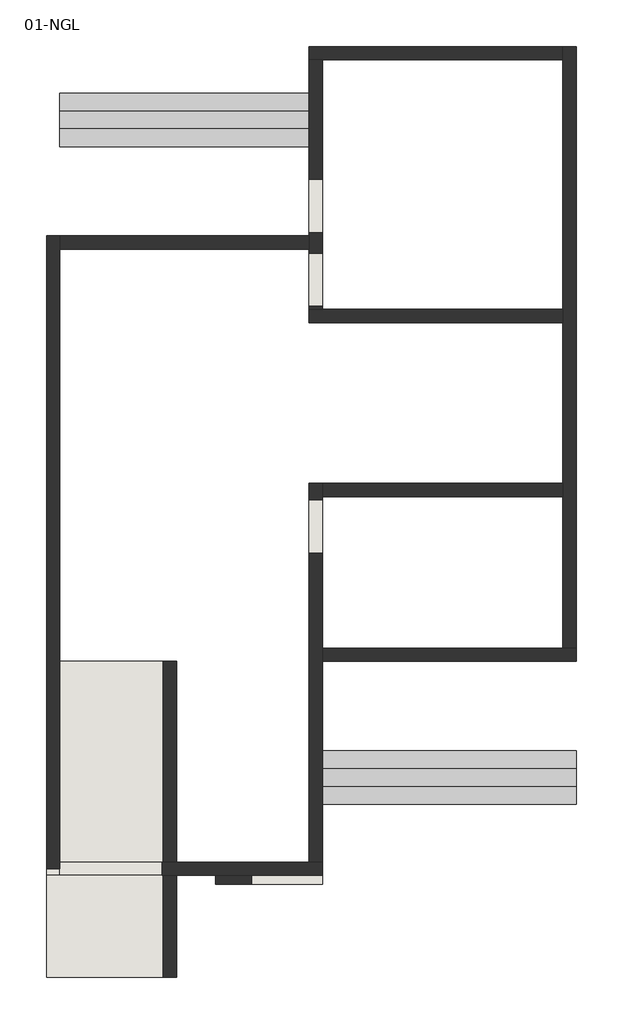
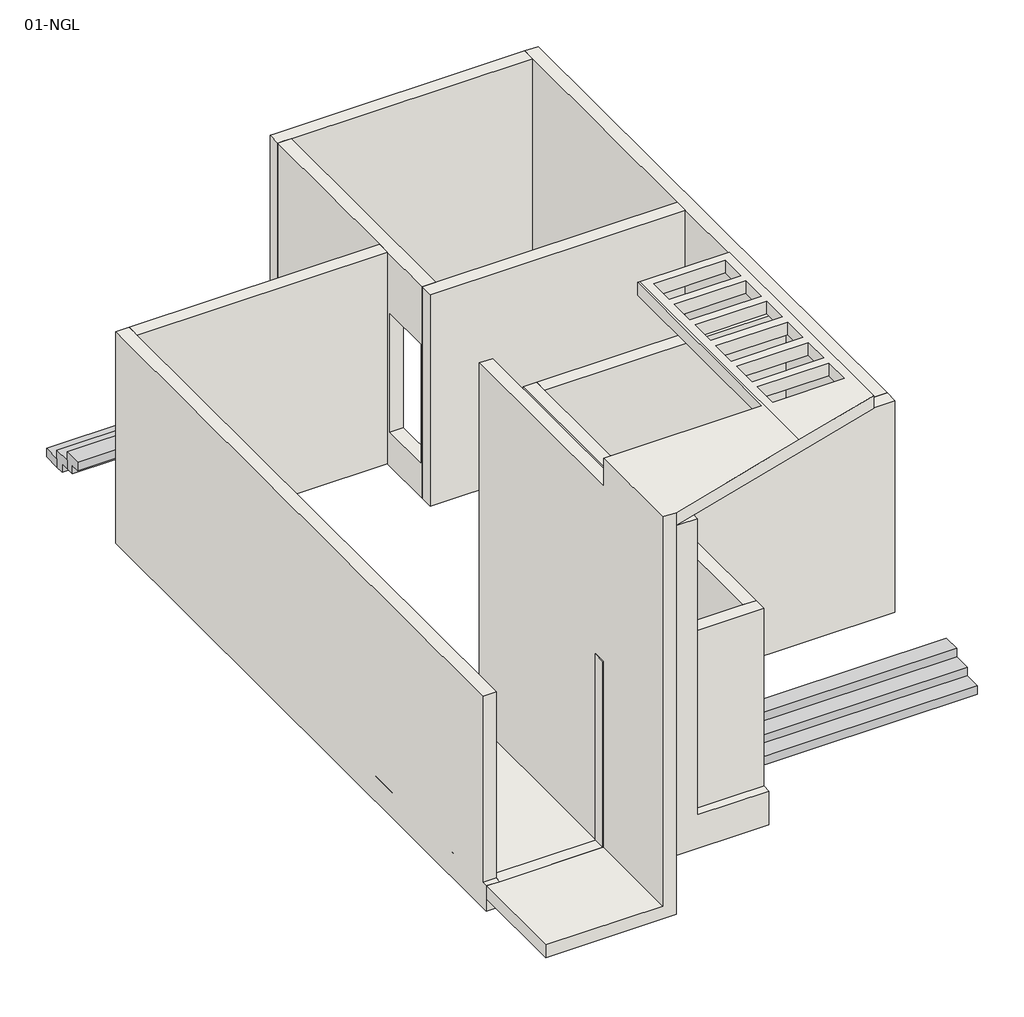
# One storey: 12 walls, 2 stair flights.
"""IFC4 building model written with IfcOpenShell, lengths in millimetres."""

from ifc_helpers import new_model, si_unit, origin, origin_with_axes, place, context, project, spatial, polyline, outline, extrude, faceted_brep, transform, mapped, element, save
from components import walls_1_walls_1_280b9ad2

model = new_model("IFC4")

# Units and contexts
model_context = context("Model", 3, world=origin())
ifc_project = project(units=[si_unit("LENGTHUNIT", "METRE", prefix="MILLI")], contexts=[model_context])

# Site, building, storey
site = spatial("IfcSite", under=ifc_project)
building = spatial("IfcBuilding", under=site)
storey = spatial("IfcBuildingStorey", under=building, Name="01-NGL", Elevation=0.0)

# Stair flights
placement = place(None, origin())
element("IfcStairFlight", 1, ObjectType="01-steps", at=placement, inside=storey, context=model_context, shape_type="Brep", body=[
    faceted_brep([(-9917.6792561, -4576.7197682, 150.0), (-9917.6792561, -4876.7197682, 150.0), (-5642.6792561, -4876.7197682, 150.0), (-5642.6792561, -4576.7197682, 150.0), (-9917.6792561, -4576.7197682, 0.0), (-9917.6792561, -4876.7197682, 0.0), (-5642.6792561, -4876.7197682, 0.0), (-5642.6792561, -4576.7197682, 0.0), (-9917.6792561, -4276.7197682, 300.0), (-9917.6792561, -4576.7197682, 300.0), (-5642.6792561, -4576.7197682, 300.0), (-5642.6792561, -4276.7197682, 300.0), (-9917.6792561, -4276.7197682, 150.0), (-9917.6792561, -4426.7197682, 150.0), (-9917.6792561, -4426.7197682, 0.0), (-5642.6792561, -4426.7197682, 0.0), (-5642.6792561, -4426.7197682, 150.0), (-5642.6792561, -4276.7197682, 150.0), (-9917.6792561, -3976.7197682, 450.0), (-9917.6792561, -4276.7197682, 450.0), (-5642.6792561, -4276.7197682, 450.0), (-5642.6792561, -3976.7197682, 450.0), (-9917.6792561, -3976.7197682, 300.0), (-9917.6792561, -4126.7197682, 300.0), (-9917.6792561, -4126.7197682, 150.0), (-5642.6792561, -4126.7197682, 150.0), (-5642.6792561, -4126.7197682, 300.0), (-5642.6792561, -3976.7197682, 300.0)], [[[0, 1, 2, 3]], [[1, 0, 4, 5]], [[2, 1, 5, 6]], [[3, 2, 6, 7]], [[8, 9, 10, 11]], [[4, 0, 9, 8, 12, 13, 14]], [[0, 3, 10, 9]], [[3, 7, 15, 16, 17, 11, 10]], [[18, 19, 20, 21]], [[19, 18, 22, 23, 24, 12, 8]], [[8, 11, 20, 19]], [[21, 20, 11, 17, 25, 26, 27]], [[18, 21, 27, 22]], [[5, 4, 14, 15, 7, 6]], [[13, 16, 15, 14]], [[24, 25, 17, 16, 13, 12]], [[25, 24, 23, 26]], [[26, 23, 22, 27]]]),
])
element("IfcStairFlight", 2, ObjectType="01-steps", at=placement, inside=storey, context=model_context, shape_type="Brep", body=[
    faceted_brep([(-10142.6792561, 6788.2802318, 150.0), (-10142.6792561, 7088.2802318, 150.0), (-14342.6792561, 7088.2802318, 150.0), (-14342.6792561, 6788.2802318, 150.0), (-14342.6792561, 7088.2802318, 0.0), (-14342.6792561, 6788.2802318, 0.0), (-10142.6792561, 7088.2802318, 0.0), (-10142.6792561, 6788.2802318, 0.0), (-10142.6792561, 6488.2802318, 300.0), (-10142.6792561, 6788.2802318, 300.0), (-14342.6792561, 6788.2802318, 300.0), (-14342.6792561, 6488.2802318, 300.0), (-14342.6792561, 6638.2802318, 0.0), (-14342.6792561, 6638.2802318, 150.0), (-14342.6792561, 6488.2802318, 150.0), (-10142.6792561, 6488.2802318, 150.0), (-10142.6792561, 6638.2802318, 150.0), (-10142.6792561, 6638.2802318, 0.0), (-10142.6792561, 6188.2802318, 450.0), (-10142.6792561, 6488.2802318, 450.0), (-14342.6792561, 6488.2802318, 450.0), (-14342.6792561, 6188.2802318, 450.0), (-14342.6792561, 6338.2802318, 150.0), (-14342.6792561, 6338.2802318, 300.0), (-14342.6792561, 6188.2802318, 300.0), (-10142.6792561, 6188.2802318, 300.0), (-10142.6792561, 6338.2802318, 300.0), (-10142.6792561, 6338.2802318, 150.0)], [[[0, 1, 2, 3]], [[3, 2, 4, 5]], [[2, 1, 6, 4]], [[1, 0, 7, 6]], [[8, 9, 10, 11]], [[3, 5, 12, 13, 14, 11, 10]], [[0, 3, 10, 9]], [[7, 0, 9, 8, 15, 16, 17]], [[18, 19, 20, 21]], [[21, 20, 11, 14, 22, 23, 24]], [[8, 11, 20, 19]], [[19, 18, 25, 26, 27, 15, 8]], [[18, 21, 24, 25]], [[6, 7, 17, 12, 5, 4]], [[16, 13, 12, 17]], [[27, 22, 14, 13, 16, 15]], [[22, 27, 26, 23]], [[23, 26, 25, 24]]]),
])

# Walls
element("IfcWall", 3, ObjectType="01-225 WALL", at=placement, inside=storey, context=model_context, shape_type="Brep", body=[
    faceted_brep([(-14567.6792561, 4688.2802318, 3750.0), (-14567.6792561, 4688.2802318, 3300.0), (-14567.6792561, 4688.2802318, 0.0), (-14567.6792561, -6069.2197682, 0.0), (-14567.6792561, -6069.2197682, 450.0), (-14567.6792561, -5964.2197682, 450.0), (-14567.6792561, -5964.2197682, 3750.0), (-14567.6792561, -5851.7197682, 3750.0), (-14567.6792561, 4575.7802318, 3750.0), (-14342.6792561, 4688.2802318, 0.0), (-14342.6792561, 4688.2802318, 3300.0), (-14342.6792561, 4688.2802318, 3750.0), (-14342.6792561, 4575.7802318, 3750.0), (-14342.6792561, 4463.2802318, 3750.0), (-14342.6792561, -5851.7197682, 3750.0), (-14342.6792561, -5964.2197682, 3750.0), (-14342.6792561, -5964.2197682, 450.0), (-14342.6792561, -6069.2197682, 450.0), (-14342.6792561, -6069.2197682, 0.0), (-14342.6792561, -5859.2197682, 0.0), (-14342.6792561, 4463.2802318, 0.0)], [[[0, 1, 2, 3, 4, 5, 6, 7, 8]], [[9, 10, 11, 12, 13, 14, 15, 16, 17, 18, 19, 20]], [[3, 2, 9, 20, 19, 18]], [[0, 8, 7, 6, 15, 14, 13, 12, 11]], [[0, 11, 10, 9, 2, 1]], [[6, 5, 16, 15]], [[16, 5, 4, 17]], [[4, 3, 18, 17]]]),
])
element("IfcWall", 4, ObjectType="01-225 WALL", at=placement, inside=storey, context=model_context, shape_type="Brep", body=[
    faceted_brep([(-12617.6792561, -6076.7197682, 0.0), (-9917.6792561, -6076.7197682, 0.0), (-9917.6792561, -6076.7197682, 3750.0), (-12617.6792561, -6076.7197682, 3750.0), (-12617.6792561, -5851.7197682, 0.0), (-12617.6792561, -5851.7197682, 450.0), (-12617.6792561, -5851.7197682, 3750.0), (-10142.6792561, -5851.7197682, 3750.0), (-9917.6792561, -5851.7197682, 3750.0), (-9917.6792561, -5851.7197682, 0.0), (-10142.6792561, -5851.7197682, 0.0)], [[[0, 1, 2, 3]], [[4, 5, 6, 7, 8, 9, 10]], [[1, 0, 4, 10, 9]], [[3, 2, 8, 7, 6]], [[2, 1, 9, 8]], [[0, 3, 6, 5, 4]]]),
])
element("IfcWall", 5, ObjectType="01-225 WALL", at=placement, inside=storey, context=model_context, shape_type="Brep", body=[
    faceted_brep([(-9917.6792561, -5851.7197682, 0.0), (-9917.6792561, -2476.7197682, 0.0), (-9917.6792561, -2251.7197682, 0.0), (-9917.6792561, 298.2802318, 0.0), (-9917.6792561, 523.2802318, 0.0), (-9917.6792561, 523.2802318, 3750.0), (-9917.6792561, 298.2802318, 3750.0), (-9917.6792561, -2251.7197682, 3750.0), (-9917.6792561, -2476.7197682, 3750.0), (-9917.6792561, -5851.7197682, 3750.0), (-9917.6792561, 248.2802318, 600.0), (-9917.6792561, -651.7197682, 600.0), (-9917.6792561, -651.7197682, 2700.0), (-9917.6792561, 248.2802318, 2700.0), (-10142.6792561, -5851.7197682, 0.0), (-10142.6792561, -5851.7197682, 3750.0), (-10142.6792561, 523.2802318, 3750.0), (-10142.6792561, 523.2802318, 0.0), (-10142.6792561, 248.2802318, 600.0), (-10142.6792561, 248.2802318, 2700.0), (-10142.6792561, -651.7197682, 2700.0), (-10142.6792561, -651.7197682, 600.0)], [[[0, 1, 2, 3, 4, 5, 6, 7, 8, 9], [10, 11, 12, 13]], [[14, 15, 16, 17], [18, 19, 20, 21]], [[4, 3, 2, 1, 0, 14, 17]], [[9, 8, 7, 6, 5, 16, 15]], [[0, 9, 15, 14]], [[5, 4, 17, 16]], [[19, 18, 10, 13]], [[20, 19, 13, 12]], [[21, 20, 12, 11]], [[18, 21, 11, 10]]]),
])
element("IfcWall", 6, ObjectType="01-225 WALL", at=placement, inside=storey, context=model_context, shape_type="Brep", body=[
    faceted_brep([(-9917.6792561, -2476.7197682, 0.0), (-5642.6792561, -2476.7197682, 0.0), (-5642.6792561, -2476.7197682, 3750.0), (-9917.6792561, -2476.7197682, 3750.0), (-9917.6792561, -2251.7197682, 0.0), (-9917.6792561, -2251.7197682, 3750.0), (-5867.6792561, -2251.7197682, 3750.0), (-5642.6792561, -2251.7197682, 3750.0), (-5642.6792561, -2251.7197682, 0.0), (-5867.6792561, -2251.7197682, 0.0)], [[[0, 1, 2, 3]], [[4, 5, 6, 7, 8, 9]], [[1, 0, 4, 9, 8]], [[3, 2, 7, 6, 5]], [[0, 3, 5, 4]], [[2, 1, 8, 7]]]),
])
element("IfcWall", 7, ObjectType="01-225 WALL", at=placement, inside=storey, context=model_context, shape_type="Brep", body=[
    faceted_brep([(-5642.6792561, -2251.7197682, 0.0), (-5642.6792561, 7873.2802318, 0.0), (-5642.6792561, 7873.2802318, 3750.0), (-5642.6792561, -2251.7197682, 3750.0), (-5867.6792561, -2251.7197682, 0.0), (-5867.6792561, -2251.7197682, 3750.0), (-5867.6792561, 298.2802318, 3750.0), (-5867.6792561, 523.2802318, 3750.0), (-5867.6792561, 3223.2802318, 3750.0), (-5867.6792561, 3448.2802318, 3750.0), (-5867.6792561, 7648.2802318, 3750.0), (-5867.6792561, 7873.2802318, 3750.0), (-5867.6792561, 7873.2802318, 0.0), (-5867.6792561, 7648.2802318, 0.0), (-5867.6792561, 3448.2802318, 0.0), (-5867.6792561, 3223.2802318, 0.0), (-5867.6792561, 523.2802318, 0.0), (-5867.6792561, 298.2802318, 0.0)], [[[0, 1, 2, 3]], [[4, 5, 6, 7, 8, 9, 10, 11, 12, 13, 14, 15, 16, 17]], [[1, 0, 4, 17, 16, 15, 14, 13, 12]], [[3, 2, 11, 10, 9, 8, 7, 6, 5]], [[0, 3, 5, 4]], [[2, 1, 12, 11]]]),
])
element("IfcWall", 8, ObjectType="01-225 WALL", at=placement, inside=storey, context=model_context, shape_type="Brep", body=[
    faceted_brep([(-5867.6792561, 7873.2802318, 0.0), (-10142.6792561, 7873.2802318, 0.0), (-10142.6792561, 7873.2802318, 3300.0), (-10142.6792561, 7873.2802318, 3750.0), (-10030.1792561, 7873.2802318, 3750.0), (-5867.6792561, 7873.2802318, 3750.0), (-5867.6792561, 7648.2802318, 0.0), (-5867.6792561, 7648.2802318, 3750.0), (-9917.6792561, 7648.2802318, 3750.0), (-10030.1792561, 7648.2802318, 3750.0), (-10142.6792561, 7648.2802318, 3750.0), (-10142.6792561, 7648.2802318, 3300.0), (-10142.6792561, 7648.2802318, 0.0), (-9917.6792561, 7648.2802318, 0.0)], [[[0, 1, 2, 3, 4, 5]], [[6, 7, 8, 9, 10, 11, 12, 13]], [[1, 0, 6, 13, 12]], [[5, 4, 3, 10, 9, 8, 7]], [[0, 5, 7, 6]], [[1, 12, 11, 10, 3, 2]]]),
])
element("IfcWall", 9, ObjectType="01-225 WALL", at=placement, inside=storey, context=model_context, shape_type="SweptSolid", body=[
    extrude(outline(polyline([(-14342.6792561, 4688.2802318), (-10142.6792561, 4688.2802318), (-10142.6792561, 4463.2802318), (-14342.6792561, 4463.2802318), (-14342.6792561, 4688.2802318)])), origin_with_axes(), (0.0, 0.0, 1.0), 3750.0),
])
element("IfcWall", 10, ObjectType="01-225 WALL", at=placement, inside=storey, context=model_context, shape_type="SweptSolid", body=[
    extrude(outline(polyline([(-5867.6792561, 298.2802318), (-9917.6792561, 298.2802318), (-9917.6792561, 523.2802318), (-5867.6792561, 523.2802318), (-5867.6792561, 298.2802318)])), origin_with_axes(), (0.0, 0.0, 1.0), 3750.0),
])
element("IfcWall", 11, ObjectType="01-225 WALL", at=placement, inside=storey, context=model_context, shape_type="Brep", body=[
    faceted_brep([(-10142.6792561, 3223.2802318, 0.0), (-5867.6792561, 3223.2802318, 0.0), (-5867.6792561, 3223.2802318, 3750.0), (-10142.6792561, 3223.2802318, 3750.0), (-10142.6792561, 3448.2802318, 0.0), (-10142.6792561, 3448.2802318, 3750.0), (-9917.6792561, 3448.2802318, 3750.0), (-5867.6792561, 3448.2802318, 3750.0), (-5867.6792561, 3448.2802318, 0.0), (-9917.6792561, 3448.2802318, 0.0)], [[[0, 1, 2, 3]], [[4, 5, 6, 7, 8, 9]], [[1, 0, 4, 9, 8]], [[3, 2, 7, 6, 5]], [[2, 1, 8, 7]], [[0, 3, 5, 4]]]),
])
element("IfcWall", 12, ObjectType="01-225 WALL", at=placement, inside=storey, context=model_context, shape_type="Brep", body=[
    faceted_brep([(-9917.6792561, 3448.2802318, 0.0), (-9917.6792561, 7648.2802318, 0.0), (-9917.6792561, 7648.2802318, 3750.0), (-9917.6792561, 3448.2802318, 3750.0), (-9917.6792561, 3498.2802318, 2700.0), (-9917.6792561, 4398.2802318, 2700.0), (-9917.6792561, 4398.2802318, 600.0), (-9917.6792561, 3498.2802318, 600.0), (-9917.6792561, 4738.2802318, 600.0), (-9917.6792561, 4738.2802318, 2700.0), (-9917.6792561, 5638.2802318, 2700.0), (-9917.6792561, 5638.2802318, 600.0), (-10142.6792561, 7648.2802318, 0.0), (-10142.6792561, 4688.2802318, 0.0), (-10142.6792561, 4463.2802318, 0.0), (-10142.6792561, 3448.2802318, 0.0), (-10142.6792561, 3448.2802318, 3750.0), (-10142.6792561, 4463.2802318, 3750.0), (-10142.6792561, 4688.2802318, 3750.0), (-10142.6792561, 7648.2802318, 3750.0), (-10142.6792561, 4398.2802318, 2700.0), (-10142.6792561, 3498.2802318, 2700.0), (-10142.6792561, 3498.2802318, 600.0), (-10142.6792561, 4398.2802318, 600.0), (-10142.6792561, 4738.2802318, 2700.0), (-10142.6792561, 4738.2802318, 600.0), (-10142.6792561, 5638.2802318, 600.0), (-10142.6792561, 5638.2802318, 2700.0)], [[[0, 1, 2, 3], [4, 5, 6, 7], [8, 9, 10, 11]], [[12, 13, 14, 15, 16, 17, 18, 19], [20, 21, 22, 23], [24, 25, 26, 27]], [[1, 0, 15, 14, 13, 12]], [[3, 2, 19, 18, 17, 16]], [[0, 3, 16, 15]], [[4, 21, 20, 5]], [[5, 20, 23, 6]], [[6, 23, 22, 7]], [[21, 4, 7, 22]], [[9, 8, 25, 24]], [[10, 9, 24, 27]], [[11, 10, 27, 26]], [[8, 11, 26, 25]], [[1, 12, 19, 2]]]),
])
element("IfcWall", 13, ObjectType="01-225 WALL MAIN", at=placement, inside=storey, context=model_context, shape_type="Brep", body=[
    faceted_brep([(-12617.6792561, -5859.2197682, 0.0), (-14342.6792561, -5859.2197682, 0.0), (-14342.6792561, -5859.2197682, 450.0), (-12617.6792561, -5859.2197682, 450.0), (-12617.6792561, -6069.2197682, 0.0), (-12617.6792561, -6069.2197682, 450.0), (-14342.6792561, -6069.2197682, 450.0), (-14342.6792561, -6069.2197682, 0.0), (-14342.6792561, -5964.2197682, 450.0)], [[[0, 1, 2, 3]], [[4, 5, 6, 7]], [[1, 0, 4, 7]], [[3, 2, 8, 6, 5]], [[0, 3, 5, 4]], [[2, 1, 7, 6, 8]]]),
])
walls_1_walls_1_shape = walls_1_walls_1_280b9ad2(model_context)
element("IfcWall", 14, ObjectType="Walls 1 : Walls 1", at=placement, inside=storey, context=model_context, shape_type="MappedRepresentation", body=[
    mapped(walls_1_walls_1_shape, transform((0.0, 0.0, 0.0), x_axis=(1.0, 0.0, 0.0), y_axis=(0.0, 1.0, 0.0), z_axis=(0.0, 0.0, 1.0))),
])

save(model, "model.ifc")

# Revit data of these elements
# Type "01-225 WALL"
#   Description = "Generic Wall (Material By Category), 200mm thick"
#   Assembly Code = "B2010"
#   Type Mark = "G06"
#   Layers, outside or top first: 225 mm no material (function 1)
# Type "01-225 WALL MAIN"
#   Description = "Generic Wall (Material By Category), 200mm thick"
#   Assembly Code = "B2010"
#   Type Mark = "G06"
#   Layers, outside or top first: 5 mm "01-WHITE WALL PAINT" (function 4); 200 mm "01-DEFAULT WALL" (function 1); 5 mm "01-WHITE WALL PAINT" (function 5)
# Elements 1, 2 (IfcStairFlight, "01-steps")
#   Phase Created = New Construction
# Element 3 (IfcWall, "01-225 WALL")
#   Top Offset = 0 mm
#   Base Offset = 0 mm
#   wall height = 3750 mm
#   Phase Created = New Construction
#   Base Constraint = 01-NGL
#   Top Constraint = 04-FIRST FLOOR
#   Materials on its faces: "Default Wall", "01-WHITE WALL PAINT"
# Elements 4, 5, 6, 7, 8, 9, 10, 11, 12 (IfcWall, "01-225 WALL")
#   Top Offset = 0 mm
#   Base Offset = 0 mm
#   wall height = 3750 mm
#   Phase Created = New Construction
#   Base Constraint = 01-NGL
#   Top Constraint = 04-FIRST FLOOR
#   Materials on its faces: "Default Wall"
# Element 13 (IfcWall, "01-225 WALL MAIN")
#   Top Offset = -150 mm
#   Base Offset = 0 mm
#   wall height = 450 mm
#   Phase Created = New Construction
#   Base Constraint = 01-NGL
#   Top Constraint = 02-DPC
#   Materials on its faces: "Default Wall", "01-WHITE WALL PAINT"
# Element 14 (IfcWall, "Walls 1 : Walls 1")
#   Phase Created = New Construction
#   Materials on its faces: "00-white plaster", "00-white plaster(2)"
# Materials
#   "01-WHITE WALL PAINT": class "Generic", colour RGB 242 242 255, transparency 0, Description = "Acoustic Ceiling Tile 24 x 48", Cost = 0
#   "01-DEFAULT WALL": class "Generic", colour RGB 242 242 255, transparency 0, Description = "Acoustic Ceiling Tile 24 x 48", Cost = 0
#   "Default Wall": colour RGB 192 192 192, transparency 0, Cost = 0
#   "00-white plaster": class "Masonry", colour RGB 244 244 244, transparency 0, Description = "Common brick", Cost = 0
#   "00-white plaster(2)": class "Masonry", colour RGB 20 28 51, transparency 0, Description = "Common brick", Cost = 0
